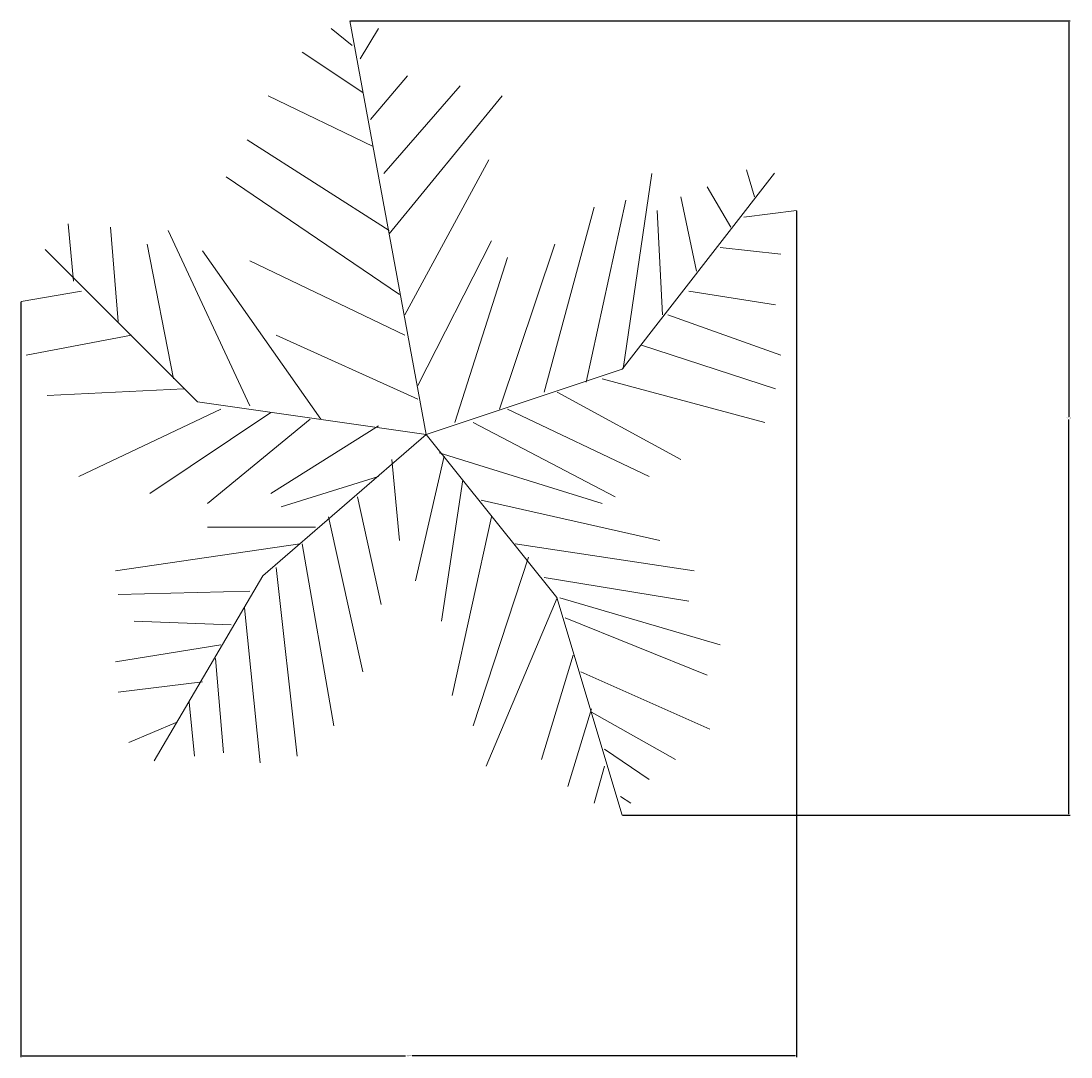
# Model space of a CAD drawing. Units: inches. Extents: x -52 to 1967, y 32 to 824.
# Tile 6 of 10: x 1295 to 1440, y 502 to 645. Entities that reach past the tile are written whole.
import ezdxf

# ---------------------------------------------------------------- set-up
doc = ezdxf.new("R2010")
doc.units = ezdxf.units.IN
doc.layers.add('A-ANNO-DIMS', color=2, linetype='Continuous', lineweight=18)
doc.layers.add('L-PLNT', color=94, linetype='Continuous', lineweight=18)
doc.styles.get("Standard").update_dxf_attribs({"font": 'arial.ttf'})
doc.dimstyles.get("Standard").update_dxf_attribs({"dimtxt": 0.18, "dimasz": 0.18, "dimexe": 0.18, "dimexo": 0.0625, "dimgap": 0.09, "dimtad": 0, "dimtih": 1, "dimtoh": 1, "dimdec": 4, "dimzin": 0, "dimdsep": 46, "dimtxsty": 'Standard', "dimcen": 0.09, "dimadec": 0, "dimazin": 0, "dimtfac": 1, "dimtdec": 4, "dimtofl": 0, "dimtmove": 0, "dimatfit": 3, "dimfxl": 1, "dimtolj": 1, "dimtzin": 0, "dimarcsym": 0})

# ---------------------------------------------------------------- blocks, each defined once
blk = doc.blocks.new('*U14')
for p, q in [((0, 0), (-10.5, 57)), ((-10.186, 53.64), (-13.084, 55.962)), ((-9.099, 51.782), (-6.563, 55.962)), ((-8.737, 47.138), (-17.069, 52.711)), ((-7.65, 43.423), (-2.578, 49.46)), ((-5.839, 35.992), (4.667, 48.067)), ((-7.288, 39.707), (-21.778, 46.673)), ((-5.114, 27.632), (10.463, 46.673)), ((-5.114, 28.097), (-24.676, 40.636)), ((-2.941, 16.486), (8.652, 37.85)), ((44.153, 36.456), (45.239, 32.741)), ((-3.665, 19.273), (-27.574, 35.527)), ((27, 9), (48, 36)), ((27.127, 9.056), (31.112, 35.992)), ((38.719, 34.134), (41.979, 28.561)), ((22.055, 7.198), (27.489, 32.277)), ((35.096, 32.741), (37.27, 22.524)), ((16.259, 5.805), (23.142, 31.348)), ((31.836, 30.883), (32.561, 16.486)), ((43.791, 29.954), (51.036, 30.883)), ((-48.585, 21.131), (-49.309, 29.026)), ((-43.513, 28.561), (-42.427, 15.558)), ((-35.544, 28.097), (-24.314, 3.947)), ((-38.442, 26.239), (-34.819, 7.663)), ((-1.129, 6.734), (9.014, 26.704)), ((10.101, 3.483), (17.708, 26.239)), ((-31.5, 4.5), (-52.5, 25.5)), ((-14.533, 2.09), (-30.834, 25.31)), ((40.53, 25.775), (48.862, 24.846)), ((-24.314, 23.917), (-2.941, 13.7)), ((3.942, 1.625), (11.187, 24.381)), ((-47.498, 19.737), (-55.83, 18.344)), ((36.183, 19.737), (48.137, 17.88)), ((33.285, 16.486), (48.862, 10.913)), ((-40.615, 13.7), (-55.105, 10.913)), ((-20.691, 13.7), (-1.129, 4.876)), ((29.662, 12.307), (48.137, 6.269)), ((0, 0), (27, 9)), ((24.229, 7.663), (46.688, 1.625)), ((-33.37, 6.269), (-52.207, 5.34)), ((18.07, 5.805), (35.096, -3.483)), ((0, 0), (-31.5, 4.5)), ((-28.299, 3.483), (-47.86, -5.805)), ((-21.416, 3.018), (-38.079, -8.128)), ((11.187, 3.483), (30.749, -5.805)), ((-15.982, 2.09), (-30.11, -9.521)), ((6.478, 1.625), (26.04, -8.592)), ((0, 0), (-22.5, -19.5)), ((-6.563, 1.161), (-21.416, -8.128)), ((0, 0), (18, -22.5)), ((1.769, -2.555), (24.229, -9.521)), ((-4.752, -3.483), (-3.665, -14.629)), ((2.493, -3.019), (-1.491, -20.202)), ((-6.563, -5.805), (-19.967, -9.985)), ((5.029, -6.27), (2.131, -25.775)), ((-9.461, -8.592), (-6.201, -23.453)), ((7.565, -9.056), (32.198, -14.629)), ((-13.446, -11.378), (-8.737, -32.741)), ((9.014, -11.378), (3.58, -35.992)), ((-15.257, -12.772), (-30.11, -12.772)), ((-17.431, -15.094), (-42.789, -18.809)), ((-17.069, -15.094), (-12.721, -40.172)), ((12.274, -15.094), (36.907, -18.809)), ((14.085, -16.951), (6.478, -40.172)), ((-20.691, -18.345), (-17.793, -44.352)), ((-22.5, -19.5), (-37.5, -45)), ((16.259, -19.738), (36.183, -22.989)), ((-24.314, -21.596), (-42.427, -22.06)), ((18.07, -22.524), (8.289, -45.745)), ((18, -22.5), (27, -52.5)), ((18.433, -22.524), (40.53, -29.026)), ((-25.038, -23.918), (-22.865, -45.281)), ((-26.849, -26.24), (-40.253, -25.775)), ((19.157, -25.311), (38.719, -33.206)), ((-28.299, -29.026), (-42.789, -31.348)), ((-29.023, -30.884), (-27.936, -43.887)), ((20.244, -30.419), (15.897, -44.816)), ((21.331, -32.741), (39.081, -40.636)), ((-30.834, -34.135), (-42.427, -35.528)), ((-32.646, -36.921), (-31.921, -44.352)), ((22.78, -37.85), (19.519, -48.532)), ((22.78, -38.314), (34.372, -44.816)), ((-34.457, -39.708), (-40.978, -42.494)), ((24.591, -43.423), (30.749, -47.603)), ((24.591, -45.745), (23.142, -50.854)), ((26.764, -49.925), (28.213, -50.854))]:
    blk.add_line(p, q)
blk = doc.blocks.new('*D133')
at = {"layer": 'A-ANNO-DIMS', "color": 0, "lineweight": -2, "transparency": 16777216}
for p, q in [((1401.77, 618.97), (1401.77, 502.3)), ((1294.9, 606.43), (1294.9, 502.3)), ((1295.08, 502.48), (1347.88, 502.48)), ((1401.59, 502.48), (1348.79, 502.48))]:
    blk.add_line(p, q, dxfattribs=at)
at = {"layer": 'A-ANNO-DIMS', "color": 0, "transparency": 16777216}
for points in [[(1295.08, 502.51), (1295.08, 502.45), (1294.9, 502.48)], [(1401.59, 502.51), (1401.59, 502.45), (1401.77, 502.48)]]:
    blk.add_solid(points, dxfattribs=at)
at = {"layer": 'Defpoints', "color": 0, "transparency": 16777216}
for p in [(1401.77, 619.03), (1294.9, 606.49), (1401.77, 502.48)]:
    blk.add_point(p, dxfattribs=at)
at = {"layer": 'A-ANNO-DIMS', "color": 0, "transparency": 16777216, "insert": (1348.34, 502.48), "char_height": 0.18, "attachment_point": 5}
blk.add_mtext('\\A1;106.87', dxfattribs=at)
blk = doc.blocks.new('*D134')
at = {"layer": 'A-ANNO-DIMS', "color": 0, "lineweight": -2, "transparency": 16777216}
for p, q in [((1340.3, 645.15), (1439.46, 645.15)), ((1439.28, 644.97), (1439.28, 590.58)), ((1439.28, 535.83), (1439.28, 590.22)), ((1377.8, 535.65), (1439.46, 535.65))]:
    blk.add_line(p, q, dxfattribs=at)
at = {"layer": 'A-ANNO-DIMS', "color": 0, "transparency": 16777216}
for points in [[(1439.25, 644.97), (1439.31, 644.97), (1439.28, 645.15)], [(1439.25, 535.83), (1439.31, 535.83), (1439.28, 535.65)]]:
    blk.add_solid(points, dxfattribs=at)
at = {"layer": 'Defpoints', "color": 0, "transparency": 16777216}
for p in [(1340.23, 645.15), (1439.28, 645.15), (1377.73, 535.65)]:
    blk.add_point(p, dxfattribs=at)
at = {"layer": 'A-ANNO-DIMS', "color": 0, "transparency": 16777216, "insert": (1439.28, 590.4), "char_height": 0.18, "attachment_point": 5}
blk.add_mtext('\\A1;109.5', dxfattribs=at)

msp = doc.modelspace()

# ---------------------------------------------------------------- block references
at = {"layer": 'L-PLNT'}
msp.add_blockref('*U14', (1350.7345, 588.1479), dxfattribs=at)

# ---------------------------------------------------------------- dimensions: what is measured, and where the dimension line sits
at = {"layer": 'A-ANNO-DIMS'}
dim = msp.add_linear_dim(base=(1439.2805, 645.1479), p1=(1377.7345, 535.6479), p2=(1340.2345, 645.1479), angle=90, dimstyle='Standard', override={"dimdec": 1, "dimlfac": 1, "dimrnd": 0, "dimzin": 0, "dimdsep": 46, "dimlunit": 2}, dxfattribs=at)
dim.commit()
dim.dimension.update_dxf_attribs({"geometry": '*D134', "text_midpoint": (1439.2805, 590.3979)})
dim = msp.add_linear_dim(base=(1401.7705, 502.4809), p1=(1294.9045, 606.4919), p2=(1401.7705, 619.0309), dimstyle='Standard', override={"dimdec": 2, "dimlfac": 1, "dimrnd": 0, "dimzin": 0, "dimdsep": 46, "dimlunit": 2}, dxfattribs=at)
dim.commit()
dim.dimension.update_dxf_attribs({"geometry": '*D133', "text_midpoint": (1348.3375, 502.4809)})

doc.saveas('drawing.dxf')
